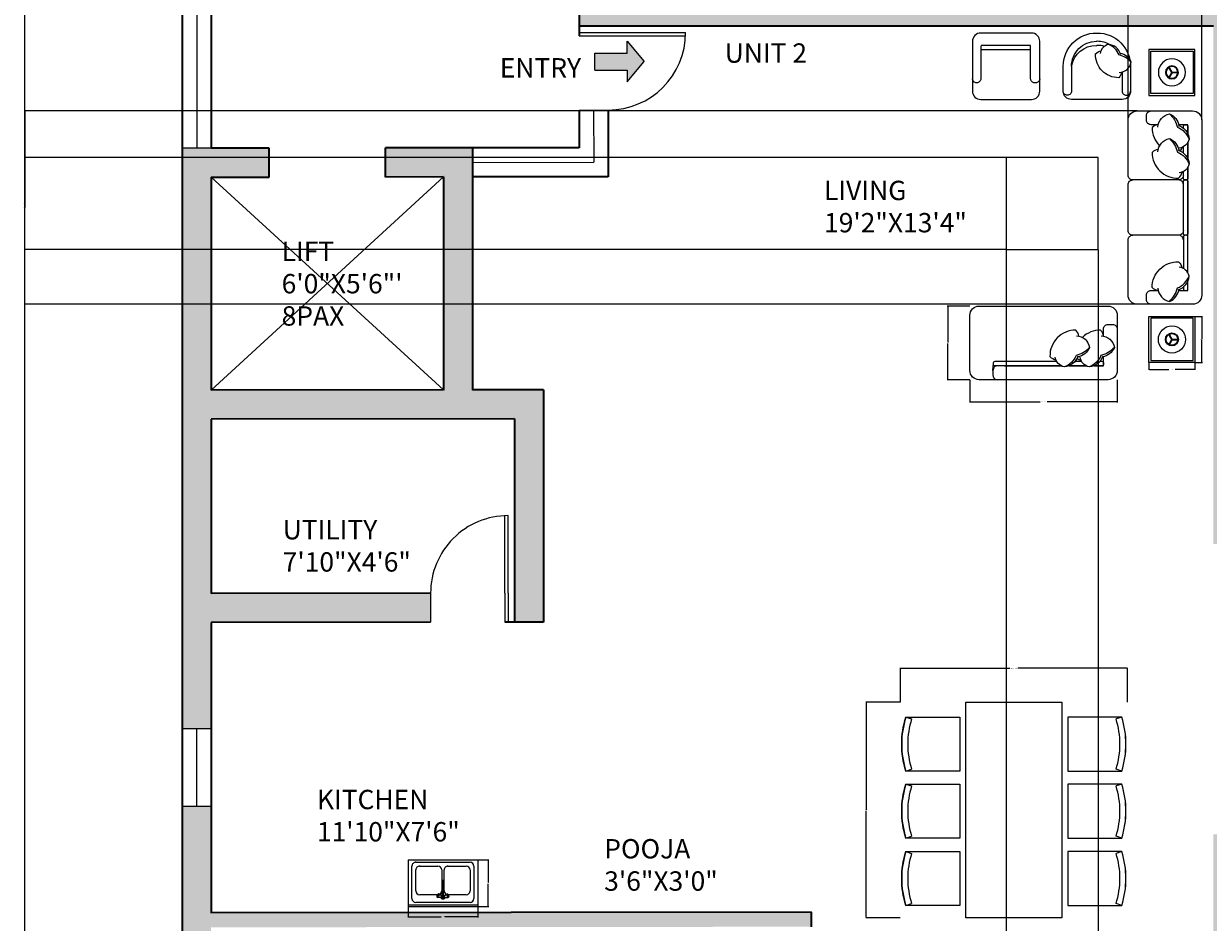
# Model space of a CAD drawing. Units: inches. Extents: x -26 to 13070, y -956 to 6917.
# Tile 2 of 13: x -26 to 341, y -744 to -466. Entities that reach past the tile are written whole.
import ezdxf

# ---------------------------------------------------------------- set-up
doc = ezdxf.new("R2010")
doc.units = ezdxf.units.IN
doc.header["$MEASUREMENT"] = 0
for name, color, linetype, lineweight in [('A-ANNO-DIMS', 2, 'Continuous', 18), ('A-ANNO-SYMB', 7, 'Continuous', 18), ('A-ANNO-TEXT', 7, 'Continuous', 18), ('A-AREA-IDEN', 7, 'Continuous', 18), ('A-DOOR', 3, 'Continuous', 18), ('A-EQPM-ELEV', 7, 'Continuous', 18), ('A-FLOR-FIXT', 9, 'Continuous', 18), ('A-FURN', 8, 'Continuous', 13), ('A-GLAZ', 4, 'Continuous', 18), ('A-WALL', 7, 'Continuous', 35), ('A-WALL-PATT', 252, 'Continuous', 13)]:
    doc.layers.add(name, color=color, linetype=linetype, lineweight=lineweight)
doc.styles.get("Standard").update_dxf_attribs({"font": 'arial.ttf'})
doc.dimstyles.get("Standard").update_dxf_attribs({"dimtxt": 0.18, "dimasz": 0.18, "dimexe": 0.18, "dimexo": 0.0625, "dimgap": 0.09, "dimtad": 0, "dimtih": 1, "dimtoh": 1, "dimdec": 0, "dimzin": 0, "dimdsep": 46, "dimlunit": 3, "dimtxsty": 'Standard', "dimcen": 0.09, "dimadec": 0, "dimazin": 0, "dimtfac": 1, "dimtdec": 0, "dimtofl": 0, "dimtmove": 0, "dimatfit": 3, "dimfxl": 1, "dimtolj": 1, "dimtzin": 0, "dimarcsym": 0})

# ---------------------------------------------------------------- blocks, each defined once
blk = doc.blocks.new('DAY BED1')
at = {"color": 0}
blk.add_line((0.3, 0.25), (0.225, 0.255), dxfattribs=at)
blk.add_lwpolyline([(-0.3, 0, -0.414214), (-0.4, 0.1), (-0.4, 0.1, 0.317837), (-0.4, 0.1, -0.414214), (-0.4, 0.1), (-0.4, 0.1, 1.186185), (-0.4, 0.1, -0.414214), (-0.4, 0.1), (-0.4, 1.5, -0.414214), (-0.3, 1.6), (0.3, 1.6, -0.414214), (0.4, 1.5), (0.4, 0.1, -0.414214), (0.3, 0)], format="xyb", close=True, dxfattribs=at)
for points in [[(-0.073, 1.45), (-0.15, 1.45, -0.414214), (-0.2, 1.5), (-0.2, 1.55, -0.414214), (-0.15, 1.6)], [(-0.076, 1.425, -0.356772), (0.05, 1.568, -0.249542), (0.154, 1.438, 9.61688)], [(0.05, 1.568, -0.14773), (0.136, 1.422, -0.213343), (0.262, 1.293, -0.178662)], [(-0.073, 1.45, 0.165541), (-0.139, 1.419, 0.200231), (-0.058, 1.221, 0.121523)], [(0.143, 1.442, -0.306663), (0.262, 1.293, -0.30633), (0.154, 1.196, 0.872847)], [(0.25, 1.345), (0.25, 1.45), (0.152, 1.45, -0.414214)], [(0.2, 1.412), (0.2, 1.43, -0.414214), (0.22, 1.45), (0.23, 1.45, -0.414214), (0.25, 1.43)], [(0.25, 1.43), (0.25, 1.345, -0.414214)], [(-0.076, 1.156, -0.356772), (0.05, 1.299, -0.249542), (0.154, 1.169, 9.61688)], [(0.05, 1.299, -0.14773), (0.136, 1.153, -0.213343), (0.262, 1.024, -0.178662)], [(-0.073, 1.181, 0.165541), (-0.139, 1.15, 0.425989), (0.148, 0.869, 0.121523), (0.187, 0.936, -7.115464)], [(0.143, 1.173, -0.306663), (0.262, 1.024, -0.30633), (0.154, 0.926, 0.872847)], [(0.168, 1.163, 0.071865), (0.187, 1.205, -7.115464)], [(0.2, 1.142), (0.2, 1.211, -0.414214)], [(0.25, 1.262), (0.25, 1.075, -0.414214)], [(0.25, 0.992), (0.25, 0.275, -0.414214), (0.23, 0.255), (0.22, 0.255, -0.414214), (0.2, 0.275), (0.2, 0.942, -0.414214)], [(0.25, 0.377), (0.25, 0.3, 0.414214), (0.3, 0.25), (0.35, 0.25, 0.414214), (0.4, 0.3)]]:
    blk.add_lwpolyline(points, format="xyb", dxfattribs=at)
for points in [[(0.25, 1.075), (0.25, 1.262)], [(0.25, 0.377), (0.25, 0.992)]]:
    blk.add_lwpolyline(points, dxfattribs=at)
blk = doc.blocks.new('М07 600х900')
for p, q in [((0, 600), (-900, 600)), ((-900, 0), (-900, 600)), ((-900, 0), (-900, 600)), ((0, 580), (-900, 580)), ((-850, 80), (-850, 500)), ((-800, 550), (-100, 550)), ((-525, 477), (-524, 480)), ((-525, 472), (-525, 477)), ((-524, 466), (-525, 472)), ((-521, 486), (-524, 480)), ((-524, 480), (-522, 481)), ((-523, 460), (-524, 466)), ((-521, 455), (-523, 460)), ((-522, 481), (-520, 481)), ((-521, 486), (-519, 487)), ((-520, 481), (-518, 479)), ((-480, 488), (-519, 487)), ((-519, 487), (-516, 487)), ((-518, 479), (-515, 475)), ((-516, 487), (-513, 484)), ((-515, 475), (-513, 470)), ((-513, 484), (-510, 479)), ((-513, 470), (-511, 464)), ((-511, 464), (-510, 458)), ((-510, 479), (-507, 473)), ((-507, 473), (-505, 465)), ((-505, 465), (-503, 458)), ((-480, 488), (-478, 487)), ((-478, 487), (-476, 486)), ((-477, 489), (-473, 496)), ((-477, 486), (-477, 489)), ((-461, 489), (-476, 485)), ((-476, 486), (-474, 483)), ((-474, 483), (-473, 479)), ((-473, 496), (-466, 503)), ((-473, 479), (-471, 474)), ((-471, 460), (-472, 459)), ((-471, 474), (-470, 470)), ((-470, 462), (-471, 460)), ((-470, 470), (-470, 466)), ((-470, 466), (-470, 462)), ((-458, 465), (-470, 462)), ((-466, 457), (-470, 461)), ((-466, 503), (-459, 507)), ((-465, 480), (-462, 489)), ((-462, 471), (-465, 480)), ((-462, 489), (-455, 494)), ((-458, 469), (-462, 471)), ((-459, 507), (-450, 508)), ((-458, 480), (-457, 485)), ((-458, 480), (-458, 280)), ((-457, 485), (-453, 488)), ((-455, 494), (-445, 494)), ((-453, 488), (-447, 488)), ((-450, 508), (-441, 507)), ((-447, 488), (-443, 485)), ((-445, 494), (-438, 489)), ((-443, 485), (-442, 480)), ((-442, 480), (-442, 280)), ((-438, 471), (-442, 469)), ((-442, 465), (-430, 462)), ((-441, 507), (-434, 503)), ((-439, 489), (-424, 485)), ((-438, 489), (-435, 480)), ((-435, 480), (-438, 471)), ((-434, 503), (-427, 496)), ((-430, 461), (-434, 457)), ((-430, 470), (-429, 474)), ((-430, 466), (-430, 470)), ((-430, 462), (-430, 466)), ((-429, 460), (-430, 462)), ((-429, 474), (-427, 479)), ((-428, 459), (-429, 460)), ((-427, 496), (-423, 489)), ((-427, 479), (-426, 483)), ((-426, 483), (-424, 486)), ((-424, 486), (-422, 487)), ((-423, 489), (-423, 486)), ((-422, 487), (-420, 488)), ((-420, 488), (-381, 487)), ((-397, 458), (-395, 465)), ((-395, 465), (-393, 473)), ((-393, 473), (-390, 479)), ((-390, 479), (-387, 484)), ((-390, 458), (-389, 464)), ((-389, 464), (-387, 470)), ((-387, 484), (-384, 487)), ((-387, 470), (-385, 475)), ((-385, 475), (-382, 479)), ((-384, 487), (-381, 487)), ((-382, 479), (-380, 481)), ((-381, 487), (-379, 486)), ((-380, 481), (-378, 481)), ((-379, 486), (-376, 480)), ((-377, 460), (-379, 455)), ((-378, 481), (-376, 480)), ((-376, 466), (-377, 460)), ((-376, 480), (-375, 477)), ((-375, 472), (-376, 466)), ((-375, 477), (-375, 472)), ((-50, 500), (-50, 80)), ((0, 0), (0, 600)), ((0, 0), (0, 600)), ((-800, 130), (-800, 400)), ((-750, 450), (-519, 450)), ((-519, 449), (-521, 455)), ((-516, 445), (-519, 449)), ((-514, 443), (-516, 445)), ((-509, 440), (-514, 443)), ((-512, 443), (-514, 443)), ((-510, 444), (-512, 443)), ((-510, 458), (-509, 452)), ((-509, 447), (-510, 444)), ((-509, 452), (-509, 447)), ((-506, 439), (-509, 440)), ((-472, 459), (-506, 439)), ((-504, 441), (-506, 439)), ((-503, 445), (-504, 441)), ((-503, 458), (-503, 451)), ((-503, 451), (-503, 445)), ((-459, 453), (-466, 457)), ((-465, 400), (-465, 130)), ((-458, 453), (-459, 453)), ((-441, 453), (-442, 453)), ((-434, 457), (-441, 453)), ((-435, 130), (-435, 400)), ((-428, 459), (-394, 439)), ((-397, 451), (-397, 458)), ((-397, 445), (-397, 451)), ((-396, 441), (-397, 445)), ((-394, 439), (-396, 441)), ((-391, 440), (-394, 439)), ((-391, 452), (-390, 458)), ((-391, 447), (-391, 452)), ((-390, 444), (-391, 447)), ((-391, 440), (-386, 443)), ((-388, 443), (-390, 444)), ((-386, 443), (-388, 443)), ((-384, 445), (-386, 443)), ((-381, 449), (-384, 445)), ((-379, 455), (-381, 449)), ((-381, 450), (-150, 450)), ((-100, 400), (-100, 130)), ((-458, 286), (-460, 280)), ((-460, 280), (-458, 274)), ((-458, 280), (-457, 275)), ((-458, 274), (-457, 270)), ((-458, 274), (-453, 271)), ((-457, 275), (-453, 272)), ((-457, 270), (-453, 267)), ((-453, 272), (-447, 272)), ((-453, 271), (-447, 271)), ((-453, 267), (-447, 267)), ((-447, 272), (-443, 275)), ((-447, 271), (-442, 274)), ((-447, 267), (-443, 270)), ((-443, 275), (-442, 280)), ((-442, 274), (-443, 270)), ((-440, 280), (-442, 286)), ((-442, 274), (-440, 280)), ((0, 0), (-900, 0)), ((-100, 30), (-800, 30)), ((-515, 80), (-750, 80)), ((-150, 80), (-385, 80))]:
    blk.add_line(p, q)
for centre, start, end in [((-800, 500), 90, 180), ((-100, 500), 0, 90), ((-750, 400), 90, 180), ((-515, 400), 0, 65.8874), ((-385, 400), 114.1126, 180), ((-150, 400), 0, 90), ((-800, 80), 180, 270), ((-750, 130), 180, 270), ((-515, 130), 270, 0), ((-385, 130), 180, 270), ((-150, 130), 270, 0), ((-100, 80), 270, 0)]:
    blk.add_arc(centre, 50, start, end)
for p in [(-515, 80), (-150, 80), (-100, 30)]:
    blk.add_point(p)
blk = doc.blocks.new('DINING-TABLE-SIX-SEATS')
for p, q in [((1.3, 62.21), (3.07, 61.65)), ((68.16, 62.21), (66.39, 61.65)), ((1.3, 45.51), (3.07, 46.07)), ((68.16, 45.51), (66.39, 46.07)), ((1.3, 41.46), (3.07, 40.9)), ((68.16, 41.46), (66.39, 40.9)), ((1.3, 24.76), (3.07, 25.32)), ((68.16, 24.76), (66.39, 25.32)), ((1.3, 20.57), (3.07, 20.01)), ((68.16, 20.57), (66.39, 20.01)), ((1.3, 3.87), (3.07, 4.43)), ((68.16, 3.87), (66.39, 4.43))]:
    blk.add_line(p, q)
blk.add_lwpolyline([(49.58, 0), (19.88, 0), (19.88, 66.83), (49.58, 66.83)], close=True)
for points in [[(1.28, 62.21), (17.99, 62.21), (17.99, 45.51), (1.28, 45.51, -0.153703), (1.28, 62.21)], [(68.17, 62.21), (51.47, 62.21), (51.47, 45.51), (68.17, 45.51, 0.153703), (68.17, 62.21)], [(1.28, 41.46), (17.99, 41.46), (17.99, 24.76), (1.28, 24.76, -0.153703), (1.28, 41.46)], [(68.17, 41.46), (51.47, 41.46), (51.47, 24.76), (68.17, 24.76, 0.153703), (68.17, 41.46)], [(1.28, 20.57), (17.99, 20.57), (17.99, 3.87), (1.28, 3.87, -0.153703), (1.28, 20.57)], [(68.17, 20.57), (51.47, 20.57), (51.47, 3.87), (68.17, 3.87, 0.153703), (68.17, 20.57)]]:
    blk.add_lwpolyline(points, format="xyb")
for centre, radius, start, end in [((27.56, 53.86), 27.56, 162.3544, 197.6456), ((27.56, 53.86), 25.7, 162.3544, 197.6456), ((41.9, 53.86), 25.7, 342.3544, 17.6456), ((41.9, 53.86), 27.56, 342.3544, 17.6456), ((27.56, 33.11), 27.56, 162.3544, 197.6456), ((27.56, 33.11), 25.7, 162.3544, 197.6456), ((41.9, 33.11), 25.7, 342.3544, 17.6456), ((41.9, 33.11), 27.56, 342.3544, 17.6456), ((27.56, 12.22), 27.56, 162.3544, 197.6456), ((27.56, 12.22), 25.7, 162.3544, 197.6456), ((41.9, 12.22), 25.7, 342.3544, 17.6456), ((41.9, 12.22), 27.56, 342.3544, 17.6456)]:
    blk.add_arc(centre, radius, start, end)
blk = doc.blocks.new('LIVING-END-TABLE')
for p, q in [((7.06, 7.09), (6.05, 8.83)), ((7.21, 7.18), (6.21, 8.92)), ((7.06, 7.18), (6.05, 5.44)), ((7.21, 7.09), (6.21, 5.35)), ((7.13, 7.22), (9.15, 7.22)), ((7.13, 7.04), (9.15, 7.04))]:
    blk.add_line(p, q)
at = {"ltscale": 0.03}
blk.add_lwpolyline([(0, 0), (0, 14.27), (14.27, 14.27), (14.27, 0)], close=True, dxfattribs=at)
blk.add_lwpolyline([(0.57, 13.7), (0.57, 0.57), (13.7, 0.57), (13.7, 13.7)], close=True)
for radius in [4.21, 2.01, 1.81]:
    blk.add_circle((7.13, 7.13), radius)
blk = doc.blocks.new('DOOR-SWING-24')
for p, q in [((24, 1), (0, 1)), ((24, 0), (0, 0))]:
    blk.add_line(p, q)
blk.add_arc((24, 0), 24, 90, 180)
blk = doc.blocks.new('WIN-24')
for p, q in [((0, 24), (0, 0)), ((9, 24), (0, 24)), ((4.5, 24), (4.5, 0)), ((9, 0), (9, 24)), ((0, 0), (9, 0))]:
    blk.add_line(p, q)
blk = doc.blocks.new('*D16')
at = {"layer": 'A-ANNO-DIMS', "color": 0, "lineweight": -2, "transparency": 16777216}
for p, q in [((322.16, -570.83), (322.16, -573.09)), ((336.43, -570.83), (336.43, -573.09)), ((322.34, -572.91), (328.33, -572.91)), ((336.25, -572.91), (330.26, -572.91))]:
    blk.add_line(p, q, dxfattribs=at)
at = {"layer": 'A-ANNO-DIMS', "color": 0, "transparency": 16777216}
for points in [[(322.34, -572.88), (322.34, -572.94), (322.16, -572.91)], [(336.25, -572.88), (336.25, -572.94), (336.43, -572.91)]]:
    blk.add_solid(points, dxfattribs=at)
at = {"layer": 'Defpoints', "color": 0, "transparency": 16777216}
for p in [(322.16, -570.77), (336.43, -570.77), (336.43, -572.91)]:
    blk.add_point(p, dxfattribs=at)
at = {"layer": 'A-ANNO-DIMS', "color": 0, "transparency": 16777216, "insert": (329.3, -572.91), "char_height": 0.18, "attachment_point": 5}
blk.add_mtext('\\A1;TABLE 14 TYP.', dxfattribs=at)
blk = doc.blocks.new('*D17')
at = {"layer": 'A-ANNO-DIMS', "color": 0, "lineweight": -2, "transparency": 16777216}
for p, q in [((336.49, -556.5), (338.75, -556.5)), ((338.57, -556.68), (338.57, -563.45)), ((338.57, -570.59), (338.57, -563.81)), ((336.49, -570.77), (338.75, -570.77))]:
    blk.add_line(p, q, dxfattribs=at)
at = {"layer": 'A-ANNO-DIMS', "color": 0, "transparency": 16777216}
for points in [[(338.54, -556.68), (338.6, -556.68), (338.57, -556.5)], [(338.54, -570.59), (338.6, -570.59), (338.57, -570.77)]]:
    blk.add_solid(points, dxfattribs=at)
at = {"layer": 'Defpoints', "color": 0, "transparency": 16777216}
for p in [(336.43, -556.5), (338.57, -556.5), (336.43, -570.77)]:
    blk.add_point(p, dxfattribs=at)
at = {"layer": 'A-ANNO-DIMS', "color": 0, "transparency": 16777216, "insert": (338.57, -563.63), "char_height": 0.18, "attachment_point": 5}
blk.add_mtext('\\A1;14 TYP.', dxfattribs=at)
blk = doc.blocks.new('*D34')
at = {"layer": 'A-ANNO-DIMS', "color": 0, "lineweight": -2, "transparency": 16777216}
for p, q in [((92.66, -739.41), (92.66, -742.76)), ((114.25, -739.41), (114.25, -742.76)), ((92.84, -742.58), (102.91, -742.58)), ((114.07, -742.58), (104, -742.58))]:
    blk.add_line(p, q, dxfattribs=at)
at = {"layer": 'A-ANNO-DIMS', "color": 0, "transparency": 16777216}
for points in [[(92.84, -742.55), (92.84, -742.61), (92.66, -742.58)], [(114.07, -742.55), (114.07, -742.61), (114.25, -742.58)]]:
    blk.add_solid(points, dxfattribs=at)
at = {"layer": 'Defpoints', "color": 0, "transparency": 16777216}
for p in [(92.66, -739.35), (114.25, -739.35), (92.66, -742.58)]:
    blk.add_point(p, dxfattribs=at)
at = {"layer": 'A-ANNO-DIMS', "color": 0, "transparency": 16777216, "insert": (103.46, -742.58), "char_height": 0.18, "attachment_point": 5}
blk.add_mtext('\\A1;SINK 22', dxfattribs=at)
blk = doc.blocks.new('*D35')
at = {"layer": 'A-ANNO-DIMS', "color": 0, "lineweight": -2, "transparency": 16777216}
for p, q in [((114.31, -724.95), (117.67, -724.95)), ((117.49, -725.13), (117.49, -731.97)), ((117.49, -739.17), (117.49, -732.33)), ((114.31, -739.35), (117.67, -739.35))]:
    blk.add_line(p, q, dxfattribs=at)
at = {"layer": 'A-ANNO-DIMS', "color": 0, "transparency": 16777216}
for points in [[(117.46, -725.13), (117.52, -725.13), (117.49, -724.95)], [(117.46, -739.17), (117.52, -739.17), (117.49, -739.35)]]:
    blk.add_solid(points, dxfattribs=at)
at = {"layer": 'Defpoints', "color": 0, "transparency": 16777216}
for p in [(114.25, -724.95), (114.25, -739.35), (117.49, -739.35)]:
    blk.add_point(p, dxfattribs=at)
at = {"layer": 'A-ANNO-DIMS', "color": 0, "transparency": 16777216, "insert": (117.49, -732.15), "char_height": 0.18, "attachment_point": 5}
blk.add_mtext('\\A1;14', dxfattribs=at)
blk = doc.blocks.new('*D36')
at = {"layer": 'A-ANNO-DIMS', "color": 0, "lineweight": -2, "transparency": 16777216}
for p, q in [((266.7, -576.18), (266.7, -583.15)), ((312.36, -576.18), (312.36, -583.15)), ((266.88, -582.97), (288.46, -582.97)), ((312.18, -582.97), (290.61, -582.97))]:
    blk.add_line(p, q, dxfattribs=at)
at = {"layer": 'A-ANNO-DIMS', "color": 0, "transparency": 16777216}
for points in [[(266.88, -582.94), (266.88, -583), (266.7, -582.97)], [(312.18, -582.94), (312.18, -583), (312.36, -582.97)]]:
    blk.add_solid(points, dxfattribs=at)
at = {"layer": 'Defpoints', "color": 0, "transparency": 16777216}
for p in [(266.7, -576.12), (312.36, -576.12), (312.36, -582.97)]:
    blk.add_point(p, dxfattribs=at)
at = {"layer": 'A-ANNO-DIMS', "color": 0, "transparency": 16777216, "insert": (289.53, -582.97), "char_height": 0.18, "attachment_point": 5}
blk.add_mtext('\\A1;DAYBED 46 TYP.', dxfattribs=at)
blk = doc.blocks.new('*D37')
at = {"layer": 'A-ANNO-DIMS', "color": 0, "lineweight": -2, "transparency": 16777216}
for p, q in [((266.64, -553.29), (259.67, -553.29)), ((259.85, -553.47), (259.85, -564.52)), ((259.85, -575.94), (259.85, -564.89)), ((266.64, -576.12), (259.67, -576.12))]:
    blk.add_line(p, q, dxfattribs=at)
at = {"layer": 'A-ANNO-DIMS', "color": 0, "transparency": 16777216}
for points in [[(259.82, -553.47), (259.88, -553.47), (259.85, -553.29)], [(259.82, -575.94), (259.88, -575.94), (259.85, -576.12)]]:
    blk.add_solid(points, dxfattribs=at)
at = {"layer": 'Defpoints', "color": 0, "transparency": 16777216}
for p in [(266.7, -553.29), (259.85, -576.12), (266.7, -576.12)]:
    blk.add_point(p, dxfattribs=at)
at = {"layer": 'A-ANNO-DIMS', "color": 0, "transparency": 16777216, "insert": (259.85, -564.7), "char_height": 0.18, "attachment_point": 5}
blk.add_mtext('\\A1;23 TYP.', dxfattribs=at)
blk = doc.blocks.new('*D38')
at = {"layer": 'A-ANNO-DIMS', "color": 0, "lineweight": -2, "transparency": 16777216}
for p, q in [((245.15, -676.04), (245.15, -665.38)), ((245.33, -665.56), (279.03, -665.56)), ((315.29, -665.56), (281.59, -665.56)), ((315.47, -676.04), (315.47, -665.38))]:
    blk.add_line(p, q, dxfattribs=at)
at = {"layer": 'A-ANNO-DIMS', "color": 0, "transparency": 16777216}
for points in [[(245.33, -665.53), (245.33, -665.59), (245.15, -665.56)], [(315.29, -665.53), (315.29, -665.59), (315.47, -665.56)]]:
    blk.add_solid(points, dxfattribs=at)
at = {"layer": 'Defpoints', "color": 0, "transparency": 16777216}
for p in [(315.47, -665.56), (245.15, -676.11), (315.47, -676.11)]:
    blk.add_point(p, dxfattribs=at)
at = {"layer": 'A-ANNO-DIMS', "color": 0, "transparency": 16777216, "insert": (280.31, -665.56), "char_height": 0.18, "attachment_point": 5}
blk.add_mtext('\\A1;DINING SET 70 TYP.', dxfattribs=at)
blk = doc.blocks.new('*D39')
at = {"layer": 'A-ANNO-DIMS', "color": 0, "lineweight": -2, "transparency": 16777216}
for p, q in [((245.08, -676.11), (234.42, -676.11)), ((234.6, -676.29), (234.6, -709.34)), ((234.6, -742.75), (234.6, -709.7)), ((245.08, -742.93), (234.42, -742.93))]:
    blk.add_line(p, q, dxfattribs=at)
at = {"layer": 'A-ANNO-DIMS', "color": 0, "transparency": 16777216}
for points in [[(234.57, -676.29), (234.63, -676.29), (234.6, -676.11)], [(234.57, -742.75), (234.63, -742.75), (234.6, -742.93)]]:
    blk.add_solid(points, dxfattribs=at)
at = {"layer": 'Defpoints', "color": 0, "transparency": 16777216}
for p in [(234.6, -676.11), (245.15, -676.11), (245.15, -742.93)]:
    blk.add_point(p, dxfattribs=at)
at = {"layer": 'A-ANNO-DIMS', "color": 0, "transparency": 16777216, "insert": (234.6, -709.52), "char_height": 0.18, "attachment_point": 5}
blk.add_mtext('\\A1;67 TYP.', dxfattribs=at)
blk = doc.blocks.new('*D41')
at = {"layer": 'A-ANNO-DIMS', "color": 0, "lineweight": -2, "transparency": 16777216}
for p, q in [((214.58, 67.46), (-26.29, 67.46)), ((-26.11, 67.28), (-26.11, -419.86)), ((-26.11, -907.36), (-26.11, -420.22)), ((208.58, -907.54), (-26.29, -907.54))]:
    blk.add_line(p, q, dxfattribs=at)
at = {"layer": 'A-ANNO-DIMS', "color": 0, "transparency": 16777216}
for points in [[(-26.14, 67.28), (-26.08, 67.28), (-26.11, 67.46)], [(-26.14, -907.36), (-26.08, -907.36), (-26.11, -907.54)]]:
    blk.add_solid(points, dxfattribs=at)
at = {"layer": 'Defpoints', "color": 0, "transparency": 16777216}
for p in [(-26.11, 67.46), (214.64, 67.46), (208.64, -907.54)]:
    blk.add_point(p, dxfattribs=at)
at = {"layer": 'A-ANNO-DIMS', "color": 0, "transparency": 16777216, "insert": (-26.11, -420.04), "char_height": 0.18, "attachment_point": 5}
blk.add_mtext('\\A1;975', dxfattribs=at)
blk = doc.blocks.new('*D49')
at = {"layer": 'A-ANNO-DIMS', "color": 0, "lineweight": -2, "transparency": 16777216}
for p, q in [((318.49, -492.81), (-26.29, -492.81)), ((-26.11, -492.99), (-26.11, -522.6)), ((-26.11, -552.57), (-26.11, -522.96)), ((318.49, -552.75), (-26.29, -552.75))]:
    blk.add_line(p, q, dxfattribs=at)
at = {"layer": 'A-ANNO-DIMS', "color": 0, "transparency": 16777216}
for points in [[(-26.14, -492.99), (-26.08, -492.99), (-26.11, -492.81)], [(-26.14, -552.57), (-26.08, -552.57), (-26.11, -552.75)]]:
    blk.add_solid(points, dxfattribs=at)
at = {"layer": 'Defpoints', "color": 0, "transparency": 16777216}
for p in [(-26.11, -492.81), (318.55, -492.81), (318.55, -552.75)]:
    blk.add_point(p, dxfattribs=at)
at = {"layer": 'A-ANNO-DIMS', "color": 0, "transparency": 16777216, "insert": (-26.11, -522.78), "char_height": 0.18, "attachment_point": 5}
blk.add_mtext('\\A1;59.93', dxfattribs=at)
blk = doc.blocks.new('*D50')
at = {"layer": 'A-ANNO-DIMS', "color": 0, "lineweight": -2, "transparency": 16777216}
for p, q in [((315.7, -495.61), (315.7, 116.39)), ((315.88, 116.21), (326.72, 116.21)), ((338.35, 116.21), (327.51, 116.21)), ((338.53, -495.61), (338.53, 116.39))]:
    blk.add_line(p, q, dxfattribs=at)
at = {"layer": 'A-ANNO-DIMS', "color": 0, "transparency": 16777216}
for points in [[(315.88, 116.24), (315.88, 116.18), (315.7, 116.21)], [(338.35, 116.24), (338.35, 116.18), (338.53, 116.21)]]:
    blk.add_solid(points, dxfattribs=at)
at = {"layer": 'Defpoints', "color": 0, "transparency": 16777216}
for p in [(338.53, 116.21), (315.7, -495.67), (338.53, -495.67)]:
    blk.add_point(p, dxfattribs=at)
at = {"layer": 'A-ANNO-DIMS', "color": 0, "transparency": 16777216, "insert": (327.12, 116.21), "char_height": 0.18, "attachment_point": 5}
blk.add_mtext('\\A1;22.83', dxfattribs=at)
blk = doc.blocks.new('*D51')
at = {"layer": 'A-ANNO-DIMS', "color": 0, "lineweight": -2, "transparency": 16777216}
for p, q in [((277.92, -535.87), (277.92, -956.47)), ((306.46, -535.87), (306.46, -956.47)), ((278.1, -956.29), (291.8, -956.29)), ((306.28, -956.29), (292.59, -956.29))]:
    blk.add_line(p, q, dxfattribs=at)
at = {"layer": 'A-ANNO-DIMS', "color": 0, "transparency": 16777216}
for points in [[(278.1, -956.26), (278.1, -956.32), (277.92, -956.29)], [(306.28, -956.26), (306.28, -956.32), (306.46, -956.29)]]:
    blk.add_solid(points, dxfattribs=at)
at = {"layer": 'Defpoints', "color": 0, "transparency": 16777216}
for p in [(277.92, -535.8), (306.46, -535.8), (306.46, -956.29)]:
    blk.add_point(p, dxfattribs=at)
at = {"layer": 'A-ANNO-DIMS', "color": 0, "transparency": 16777216, "insert": (292.19, -956.29), "char_height": 0.18, "attachment_point": 5}
blk.add_mtext('\\A1;28.54', dxfattribs=at)
blk = doc.blocks.new('*D52')
at = {"layer": 'A-ANNO-DIMS', "color": 0, "lineweight": -2, "transparency": 16777216}
for p, q in [((277.86, -507.27), (-26.29, -507.27)), ((-26.11, -507.45), (-26.11, -521.35)), ((-26.11, -535.62), (-26.11, -521.72)), ((277.86, -535.8), (-26.29, -535.8))]:
    blk.add_line(p, q, dxfattribs=at)
at = {"layer": 'A-ANNO-DIMS', "color": 0, "transparency": 16777216}
for points in [[(-26.14, -507.45), (-26.08, -507.45), (-26.11, -507.27)], [(-26.14, -535.62), (-26.08, -535.62), (-26.11, -535.8)]]:
    blk.add_solid(points, dxfattribs=at)
at = {"layer": 'Defpoints', "color": 0, "transparency": 16777216}
for p in [(-26.11, -507.27), (277.92, -507.27), (277.92, -535.8)]:
    blk.add_point(p, dxfattribs=at)
at = {"layer": 'A-ANNO-DIMS', "color": 0, "transparency": 16777216, "insert": (-26.11, -521.54), "char_height": 0.18, "attachment_point": 5}
blk.add_mtext('\\A1;28.54', dxfattribs=at)

msp = doc.modelspace()

# ---------------------------------------------------------------- hatches: boundary and pattern name
at = {"layer": 'A-ANNO-SYMB'}
h = msp.add_hatch(color=256, dxfattribs=at)
h.dxf.hatch_style = 1
h.paths.add_polyline_path([(160.337, -438.111), (160.337, -441.783), (150.328, -441.783), (150.328, -447.062), (160.337, -447.062), (160.337, -450.734), (165.598, -444.423)])
h.paths.add_polyline_path([(165.824, -477.533), (160.564, -471.221), (160.564, -474.894), (150.555, -474.894), (150.555, -480.172), (160.564, -480.172), (160.564, -483.845)])
at = {"layer": 'A-WALL-PATT'}
h = msp.add_hatch(color=256, dxfattribs=at)
h.dxf.hatch_style = 1
h.paths.add_polyline_path([(223.641, 10.458), (214.641, 10.458), (22.641, 10.458), (22.641, -171.042), (31.641, -171.042), (31.641, -135.042), (205.641, -135.042), (205.641, -241.042), (210.141, -241.042), (210.141, -130.542), (94.641, -130.542), (94.641, -76.542), (85.641, -76.542), (85.641, -126.042), (27.141, -126.042), (27.141, 5.958), (85.641, 5.958), (85.641, -52.542), (94.641, -52.542), (94.641, 1.458), (214.641, 1.458), (214.641, -16.542), (223.641, -16.542), (229.641, -16.542), (229.641, -7.542), (223.641, -7.542)])
h.paths.add_polyline_path([(367.048, 10.458), (346.641, 10.458), (337.641, 10.458), (337.641, -7.542), (331.641, -7.542), (331.641, -16.542), (337.641, -16.542), (342.141, -16.542), (342.141, -128.542), (346.641, -128.542), (346.641, 1.458), (367.048, 1.458)])
h.paths.add_polyline_path([(547.641, 10.458), (403.048, 10.458), (403.048, 1.458), (538.641, 1.458), (538.641, -46.542), (547.641, -46.542)])
h.paths.add_polyline_path([(547.641, -106.542), (538.641, -106.542), (538.641, -154.542), (481.013, -154.542), (481.013, -159.042), (538.641, -159.042), (547.641, -159.042)])
h.paths.add_polyline_path([(457.013, -154.542), (342.141, -154.542), (342.141, -165.042), (346.641, -165.042), (346.641, -159.042), (414.141, -159.042), (414.141, -225.042), (346.641, -225.042), (346.641, -189.042), (342.141, -189.042), (342.141, -234.042), (390.641, -234.042), (390.641, -286.042), (395.141, -286.042), (395.141, -234.042), (456.141, -234.042), (456.141, -312.042), (372.641, -312.042), (372.641, -316.542), (462.641, -316.542), (462.641, -312.042), (460.641, -312.042), (460.641, -234.042), (538.641, -234.042), (547.641, -234.042), (547.641, -195.042), (538.641, -195.042), (538.641, -225.042), (418.641, -225.042), (418.641, -159.042), (457.013, -159.042)])
h.paths.add_polyline_path([(547.641, -270.042), (538.641, -270.042), (538.641, -312.042), (486.641, -312.042), (486.641, -316.542), (538.641, -316.542), (547.641, -316.542)], flags=0)
h.paths.add_polyline_path([(547.641, -456.306), (538.641, -456.306), (538.641, -457.542), (346.641, -457.542), (346.641, -316.542), (346.641, -312.042), (342.141, -312.042), (342.141, -457.542), (145.641, -457.542), (145.641, -466.542), (342.141, -466.542), (342.141, -627.042), (346.641, -627.042), (346.641, -466.542), (538.641, -466.542), (538.641, -514.542), (547.641, -514.542)])
h.paths.add_polyline_path([(466.641, -622.542), (372.641, -622.542), (372.641, -627.042), (388.641, -627.042), (388.641, -721.542), (393.141, -721.542), (393.141, -627.042), (462.141, -627.042), (462.141, -717.042), (466.641, -717.042)])
h.paths.add_polyline_path([(547.641, -574.542), (538.641, -574.542), (538.641, -622.542), (492.641, -622.542), (492.641, -627.042), (538.641, -627.042), (538.641, -654.042), (547.641, -654.042)])
h.paths.add_polyline_path([(547.641, -690.042), (538.641, -690.042), (538.641, -717.042), (466.641, -717.042), (466.641, -721.542), (538.641, -721.542), (538.641, -763.542), (547.641, -763.542)])
h.paths.add_polyline_path([(462.141, -717.042), (419.141, -717.042), (419.141, -721.542), (462.141, -721.542)], flags=0)
h.paths.add_polyline_path([(346.641, -721.542), (352.641, -721.542), (352.641, -717.042), (342.141, -717.042), (342.141, -874.542), (342.141, -907.542), (351.141, -907.542), (351.141, -874.542), (395.949, -874.542), (395.949, -865.542), (351.141, -865.542), (351.141, -841.542), (346.641, -841.542)])
h.paths.add_polyline_path([(547.641, -823.542), (538.641, -823.542), (538.641, -865.542), (431.949, -865.542), (431.949, -874.542), (547.641, -874.542)])
h.paths.add_polyline_path([(172.641, -865.713), (140.641, -865.744), (140.641, -788.744), (182.646, -788.704), (182.641, -784.204), (136.141, -784.249), (136.141, -848.332), (131.641, -848.332), (131.641, -874.542), (172.641, -874.542)])
h.paths.add_polyline_path([(217.641, -816.13), (213.141, -816.13), (213.141, -784.174), (208.641, -784.179), (208.641, -865.679), (208.641, -874.542), (217.641, -874.542)])
h.paths.add_polyline_path([(95.641, -865.788), (31.641, -865.849), (31.641, -832.695), (22.641, -832.695), (22.641, -874.542), (95.641, -874.542)])
h.paths.add_polyline_path([(217.641, -741.17), (31.641, -741.349), (31.641, -708.349), (22.641, -708.349), (22.641, -772.542), (22.641, -796.695), (31.641, -796.695), (31.641, -763.542), (31.641, -745.849), (217.641, -745.67)])
h.paths.add_polyline_path([(31.641, -651.349), (99.65, -651.284), (99.641, -642.284), (31.641, -642.349), (31.641, -639.042), (31.641, -588.349), (125.641, -588.259), (125.641, -651.259), (134.641, -651.25), (134.641, -579.25), (112.641, -579.271), (112.641, -549.042), (112.641, -504.271), (85.633, -504.297), (85.641, -513.297), (103.641, -513.28), (103.641, -549.042), (103.641, -579.28), (31.641, -579.349), (31.641, -549.042), (31.641, -513.349), (49.641, -513.314), (49.633, -504.332), (31.641, -504.349), (22.641, -504.358), (22.641, -684.349), (31.641, -684.349)])
h.paths.add_polyline_path([(31.641, -276.042), (145.641, -276.042), (145.641, -402.042), (145.641, -419.542), (154.641, -419.542), (154.641, -411.042), (154.641, -271.542), (210.141, -271.542), (210.141, -265.042), (205.641, -265.042), (205.641, -267.042), (31.641, -267.042), (31.641, -231.042), (22.641, -231.042), (22.641, -426.852), (31.641, -426.852), (31.641, -411.042), (31.641, -402.042)])

# ---------------------------------------------------------------- linework, layer by layer
at = {"layer": 'A-ANNO-SYMB'}
for p, q in [((160.564, -474.894), (160.564, -471.221)), ((160.564, -471.221), (165.824, -477.533)), ((150.555, -480.172), (150.555, -474.894)), ((150.555, -474.894), (160.564, -474.894)), ((150.555, -480.172), (160.564, -480.172)), ((160.564, -483.845), (165.824, -477.533)), ((160.564, -480.172), (160.564, -483.845))]:
    msp.add_line(p, q, dxfattribs=at)
at = {"layer": 'A-DOOR'}
for p, q in [((145.641, -468.542), (154.641, -468.542)), ((145.641, -469.542), (154.641, -469.542)), ((145.641, -492.542), (154.641, -492.542)), ((122.641, -642.261), (122.641, -618.261)), ((123.641, -642.261), (123.641, -618.261)), ((99.641, -642.261), (99.65, -651.284)), ((122.641, -642.26), (122.65, -651.261)), ((123.641, -642.259), (123.65, -651.261))]:
    msp.add_line(p, q, dxfattribs=at)
msp.add_arc((123.641, -642.26), 24, 90, 180.05517, dxfattribs=at)
at = {"layer": 'A-EQPM-ELEV'}
for p, q in [((103.641, -513.28), (31.641, -579.349)), ((31.641, -513.349), (103.641, -579.28))]:
    msp.add_line(p, q, dxfattribs=at)
at = {"layer": 'A-FURN', "ltscale": 0.03}
for points in [[(270.069, -468.669), (270.069, -468.669, 0.4142136), (267.496, -471.242), (267.496, -486.682, 0.4142136), (270.069, -489.255), (270.069, -489.255), (285.766, -489.255, 0.4142136), (288.339, -486.682), (288.339, -471.242, 0.4142136), (285.766, -468.669)], [(318.554, -552.747, -0.4142136), (315.7, -549.893), (315.7, -532.769, -0.4142136), (317.127, -531.342, -0.4142136), (315.7, -529.915), (315.7, -515.646, -0.4142136), (317.127, -514.219, -0.4142136), (315.7, -512.792), (315.7, -495.668, -0.4142136), (318.554, -492.814), (335.677, -492.814, -0.4142136), (338.531, -495.668), (338.531, -549.893, -0.4142136), (335.677, -552.747)]]:
    msp.add_lwpolyline(points, format="xyb", close=True, dxfattribs=at)
msp.add_lwpolyline([(306.035, -489.255), (298.187, -489.255, -0.4142136), (295.614, -486.682), (295.614, -478.962, -0.4142136), (305.907, -468.669), (306.035, -468.669), (306.164, -468.669, -0.4142136), (316.457, -478.962), (316.457, -486.682, -0.4142136), (313.884, -489.255), (306.035, -489.255)], format="xyb", dxfattribs=at)
at = {"layer": 'A-FURN'}
for points in [[(270.069, -473.301), (270.069, -482.822, -0.4142136), (268.783, -484.109), (268.783, -484.109, -0.4142136), (267.496, -482.822)], [(280.662, -472.529), (270.584, -472.529, 0.4142136), (270.069, -473.044), (270.069, -473.301, 0.4142136), (270.584, -473.816), (279.366, -473.816, 0.4142136)], [(279.366, -473.816), (284.994, -473.816, 0.4142136), (285.509, -473.301), (285.509, -473.044, 0.4142136), (284.994, -472.529)], [(284.994, -472.529), (280.662, -472.529, 0.4142136)], [(298.187, -478.962, -0.4142136), (305.907, -471.242), (306.035, -471.242)], [(298.187, -478.962, -0.3727189), (305.907, -472.529), (306.035, -472.529)], [(309.996, -472.261, 0.1305915), (306.164, -471.242), (306.035, -471.242)], [(308.358, -472.806, 0.0723842), (306.164, -472.529), (306.035, -472.529)], [(313.427, -475.276, 0.3066635), (309.589, -472.209, 0.30633), (307.082, -475.01, -0.8728472)], [(316.668, -477.663, 0.1477299), (312.907, -475.452, 0.2133428), (309.589, -472.209, 0.1786618)], [(313.629, -480.828, -0.1655406), (312.833, -482.528, -0.4259892), (305.607, -475.157, -0.1215233), (307.323, -474.141, 7.1154643)], [(312.981, -480.906, 0.3567724), (316.668, -477.663, 0.2495421), (313.327, -474.991, -9.6168803)], [(298.187, -478.962), (298.187, -486.682, -0.4142136), (296.9, -487.968), (296.9, -487.968, -0.4142136), (295.614, -486.682)], [(288.339, -482.822, -0.4142136), (287.053, -484.109), (286.795, -484.109, -0.4142136), (285.509, -482.822), (285.509, -480.828)], [(313.884, -480.766), (313.884, -486.682, 0.4142136), (315.17, -487.968), (315.17, -487.968, 0.4142136), (316.457, -486.682)], [(325.045, -497.095), (322.835, -497.095, -0.4142136), (321.408, -495.668), (321.408, -494.241, -0.4142136), (322.835, -492.814)], [(324.959, -497.811, -0.3567724), (328.556, -493.722, -0.2495421), (331.52, -497.427, 9.6168803)], [(328.556, -493.722, -0.1477299), (331.008, -497.893, -0.2133428), (334.605, -501.573, -0.1786618)], [(325.046, -497.092, 0.1655406), (323.161, -497.975, 0.2002311), (325.457, -503.639, 0.1215233)], [(331.204, -497.317, -0.3066635), (334.605, -501.573, -0.30633), (331.499, -504.353, 0.8728472)], [(334.25, -500.097), (334.25, -497.095), (331.446, -497.095, -0.4142136)], [(332.823, -498.184), (332.823, -497.666, -0.4142136), (333.394, -497.095), (333.68, -497.095, -0.4142136), (334.25, -497.666)], [(334.25, -497.666), (334.25, -500.097, -0.4142136)], [(324.959, -505.498, -0.3567724), (328.556, -501.409, -0.2495421), (331.52, -505.114, 9.6168803)], [(328.556, -501.409, -0.1477299), (331.008, -505.58, -0.2133428), (334.605, -509.26, -0.1786618)], [(334.25, -502.471), (334.25, -507.784, -0.4142136)], [(325.046, -504.779, 0.1655406), (323.161, -505.662, 0.4259892), (331.335, -513.676, 0.1215233), (332.462, -511.773, -7.1154643)], [(331.204, -505.004, -0.3066635), (334.605, -509.26, -0.30633), (331.499, -512.04, 0.8728472)], [(331.904, -505.283, 0.0718654), (332.462, -504.086, -7.1154643)], [(332.823, -505.871), (332.823, -503.908, -0.4142136)], [(332.823, -512.792, -0.4142136), (331.396, -514.219), (317.127, -514.219, -0.4142136)], [(334.25, -510.158), (334.25, -513.648, -0.4142136), (333.68, -514.219), (333.394, -514.219, -0.4142136), (332.823, -513.648), (332.823, -511.595, -0.4142136)], [(332.823, -515.646, 0.4142136), (331.396, -514.219)], [(332.823, -532.769, 0.4142136), (331.396, -531.342), (317.127, -531.342, 0.4142136)], [(332.823, -529.915, -0.4142136), (331.396, -531.342)], [(334.25, -543.09), (334.25, -531.913, 0.4142136), (333.68, -531.342), (333.394, -531.342, 0.4142136), (332.823, -531.913), (332.823, -541.653, 0.4142136)], [(325.046, -548.469, -0.1655406), (323.161, -547.586, -0.4259892), (331.335, -539.572, -0.1215233), (332.462, -541.475, 7.1154643)], [(331.204, -548.244, 0.3066635), (334.605, -543.988, 0.30633), (331.499, -541.208, -0.8728472)], [(328.556, -551.839, 0.1477299), (331.008, -547.668, 0.2133428), (334.605, -543.988, 0.1786618)], [(334.25, -547.895), (334.25, -545.464, 0.4142136)], [(322.835, -552.747, -0.4142136), (321.408, -551.32), (321.408, -549.893, -0.4142136), (322.835, -548.466), (325.045, -548.466)], [(324.959, -547.75, 0.3567724), (328.556, -551.839, 0.2495421), (331.52, -548.134, -9.6168803)], [(332.823, -547.377), (332.823, -547.895, 0.4142136), (333.394, -548.466), (333.68, -548.466, 0.4142136), (334.25, -547.895)]]:
    msp.add_lwpolyline(points, format="xyb", dxfattribs=at)
for points in [[(280.662, -472.529), (270.198, -472.529)], [(285.509, -480.828), (285.509, -472.529), (280.662, -472.529)], [(334.25, -507.784), (334.25, -502.471)], [(334.25, -543.09), (334.25, -510.158)], [(331.446, -548.466), (334.25, -548.466), (334.25, -545.464)]]:
    msp.add_lwpolyline(points, dxfattribs=at)
at = {"layer": 'A-FURN', "ltscale": 0.03}
msp.add_lwpolyline([(277.924, -507.265), (277.924, -535.805), (306.464, -535.805), (306.464, -507.265)], close=True, dxfattribs=at)
at = {"layer": 'A-FURN'}
msp.add_lwpolyline([(334.25, -514.789), (334.25, -530.772, -0.4142136), (333.68, -531.342), (333.394, -531.342, -0.4142136), (332.823, -530.772), (332.823, -514.789, -0.4142136), (333.394, -514.219), (333.68, -514.219, -0.4142136)], format="xyb", close=True, dxfattribs=at)
at = {"layer": 'A-GLAZ'}
for p, q in [((27.141, -426.852), (27.216, -504.353)), ((150.141, -492.542), (150.157, -508.735)), ((31.641, -504.349), (22.641, -504.358)), ((112.646, -508.771), (150.157, -508.735))]:
    msp.add_line(p, q, dxfattribs=at)
at = {"layer": 'A-WALL'}
for p, q in [((22.641, 10.458), (22.641, -772.542)), ((31.641, -411.042), (31.641, -477.042)), ((145.641, -454.542), (145.641, -469.542)), ((342.141, -466.542), (145.641, -466.542)), ((31.641, -477.042), (31.641, -504.349)), ((145.641, -492.542), (145.641, -504.239)), ((154.641, -492.542), (154.641, -513.231)), ((49.633, -504.332), (31.641, -504.349)), ((49.641, -513.314), (49.633, -504.332)), ((145.641, -504.239), (85.633, -504.297)), ((85.641, -513.314), (85.633, -504.297)), ((112.641, -504.271), (112.641, -549.042)), ((31.641, -513.349), (49.641, -513.314)), ((31.641, -513.349), (31.641, -549.042)), ((103.641, -513.28), (85.641, -513.297)), ((103.641, -513.28), (103.641, -549.042)), ((154.641, -513.231), (112.641, -513.271)), ((31.641, -549.042), (31.641, -579.349)), ((103.641, -549.042), (103.641, -579.349)), ((112.641, -549.042), (112.641, -579.349)), ((103.641, -579.28), (31.641, -579.349)), ((134.641, -579.25), (112.641, -579.271)), ((134.641, -579.25), (134.641, -651.25)), ((125.641, -588.259), (31.641, -588.349)), ((31.641, -588.349), (31.641, -639.042)), ((125.641, -588.259), (125.641, -651.259)), ((31.641, -639.042), (31.641, -642.349)), ((99.641, -642.284), (31.641, -642.349)), ((99.65, -651.284), (31.641, -651.349)), ((31.641, -651.349), (31.641, -741.349)), ((134.641, -651.25), (122.65, -651.261)), ((217.641, -741.17), (31.521, -741.349)), ((217.641, -745.67), (217.641, -741.17))]:
    msp.add_line(p, q, dxfattribs=at)

# ---------------------------------------------------------------- block references
at = {"layer": 'A-DOOR', "rotation": 180}
msp.add_blockref('DOOR-SWING-24', (178.641, -468.541), dxfattribs=at)
at = {"layer": 'A-FLOR-FIXT', "xscale": 0.023991081880656, "yscale": 0.023991081880656, "zscale": 0.023991081880656, "rotation": 180}
msp.add_blockref('М07 600х900', (92.66, -724.951), dxfattribs=at)
at = {"layer": 'A-FURN', "extrusion": (0, 0, -1), "zscale": -1, "rotation": 180}
msp.add_blockref('LIVING-END-TABLE', (-322.16, -473.732), dxfattribs=at)
at = {"layer": 'A-FURN', "ltscale": 0.03, "xscale": 28.53951744329711, "yscale": 28.53951744329711, "zscale": 28.53951744329711, "rotation": 270}
msp.add_blockref('DAY BED1', (266.7, -564.704), dxfattribs=at)
at = {"layer": 'A-FURN'}
for name, p in [('LIVING-END-TABLE', (322.16, -570.765)), ('DINING-TABLE-SIX-SEATS', (245.579, -742.931))]:
    msp.add_blockref(name, p, dxfattribs=at)
at = {"layer": 'A-GLAZ'}
msp.add_blockref('WIN-24', (22.641, -708.349), dxfattribs=at)

# ---------------------------------------------------------------- texts
at = {"layer": 'A-ANNO-TEXT', "insert": (121.066, -476.456), "char_height": 6, "attachment_point": 1}
msp.add_mtext('ENTRY', dxfattribs=at)
at = {"layer": 'A-AREA-IDEN', "char_height": 6, "attachment_point": 1}
for s, insert in [('UNIT 2', (190.75, -471.885)), ('LIVING\\P19\'2"X13\'4"', (221.517, -514.456)), ('LIFT\\P6\'0"X5\'6"\'\\P8PAX', (53.496, -533.361)), ('UTILITY\\P7\'10"X4\'6"', (53.823, -619.602)), ('KITCHEN\\P11\'10"X7\'6"', (64.413, -703.234)), ('POOJA\\P3\'6"X3\'0"', (153.418, -718.502))]:
    msp.add_mtext(s, dxfattribs=dict(at, insert=insert))

# ---------------------------------------------------------------- dimensions: what is measured, and where the dimension line sits
at = {"layer": 'A-ANNO-DIMS'}
for base, p1, p2, picture, middle in [((338.531, 116.209), (315.7, -495.668), (338.531, -495.668), '*D50', (327.115, 116.209)), ((306.464, -956.293), (277.924, -535.805), (306.464, -535.805), '*D51', (292.194, -956.293))]:
    dim = msp.add_linear_dim(base=base, p1=p1, p2=p2, dimstyle='Standard', override={"dimdec": 2, "dimlfac": 1, "dimrnd": 0, "dimzin": 0, "dimdsep": 46, "dimlunit": 2}, dxfattribs=at)
    dim.commit()
    dim.dimension.update_dxf_attribs({"geometry": picture, "text_midpoint": middle})
for base, p1, p2, angle, override, picture, middle in [((-26.11, 67.458), (208.641, -907.542), (214.641, 67.458), 90, {"dimdec": 0, "dimlfac": 1, "dimrnd": 0, "dimzin": 0, "dimdsep": 46, "dimlunit": 2}, '*D41', (-26.11, -420.042)), ((-26.11, -492.814), (318.554, -552.747), (318.554, -492.814), 90, {"dimdec": 2, "dimlfac": 1, "dimrnd": 0, "dimzin": 0, "dimdsep": 46, "dimlunit": 2}, '*D49', (-26.11, -522.781)), ((-26.11, -507.265), (277.924, -535.805), (277.924, -507.265), 90, {"dimdec": 2, "dimlfac": 1, "dimrnd": 0, "dimzin": 0, "dimdsep": 46, "dimlunit": 2}, '*D52', (-26.11, -521.535)), ((117.491, -739.346), (114.252, -724.951), (114.252, -739.346), 270, {"dimdec": 0, "dimlfac": 1, "dimrnd": 0, "dimzin": 0, "dimdsep": 46, "dimlunit": 2}, '*D35', (117.491, -732.149))]:
    dim = msp.add_linear_dim(base=base, p1=p1, p2=p2, angle=angle, dimstyle='Standard', override=override, dxfattribs=at)
    dim.commit()
    dim.dimension.update_dxf_attribs({"geometry": picture, "text_midpoint": middle})
for base, p1, p2, angle, text, picture, middle in [((259.85, -576.12), (266.7, -553.288), (266.7, -576.12), 270, '<> TYP.', '*D37', (259.85, -564.704)), ((338.571, -556.496), (336.43, -570.766), (336.43, -556.496), 90, '<> TYP.', '*D17', (338.571, -563.631)), ((234.599, -676.106), (245.147, -742.931), (245.147, -676.106), 90, '<> TYP.', '*D39', (234.599, -709.518)), ((92.66, -742.585), (114.252, -739.346), (92.66, -739.346), 180, 'SINK <>', '*D34', (103.456, -742.585))]:
    dim = msp.add_linear_dim(base=base, p1=p1, p2=p2, angle=angle, text=text, dimstyle='Standard', override={"dimdec": 0, "dimlfac": 1, "dimrnd": 0, "dimzin": 0, "dimdsep": 46, "dimlunit": 2}, dxfattribs=at)
    dim.commit()
    dim.dimension.update_dxf_attribs({"geometry": picture, "text_midpoint": middle})
for base, p1, p2, text, picture, middle in [((336.43, -572.906), (322.16, -570.766), (336.43, -570.766), 'TABLE <> TYP.', '*D16', (329.295, -572.906)), ((312.363, -582.969), (266.7, -576.12), (312.363, -576.12), 'DAYBED <> TYP.', '*D36', (289.531, -582.969)), ((315.467, -665.558), (245.147, -676.106), (315.467, -676.106), 'DINING SET <> TYP.', '*D38', (280.307, -665.558))]:
    dim = msp.add_linear_dim(base=base, p1=p1, p2=p2, text=text, dimstyle='Standard', override={"dimdec": 0, "dimlfac": 1, "dimrnd": 0, "dimzin": 0, "dimdsep": 46, "dimlunit": 2}, dxfattribs=at)
    dim.commit()
    dim.dimension.update_dxf_attribs({"geometry": picture, "text_midpoint": middle})

doc.saveas('drawing.dxf')
